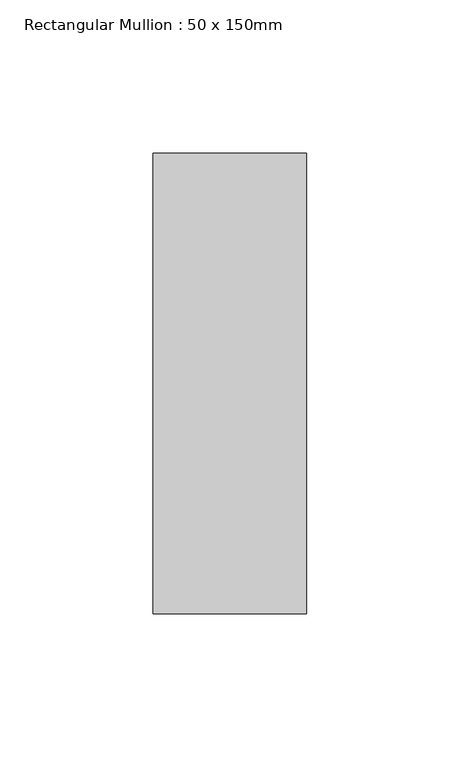
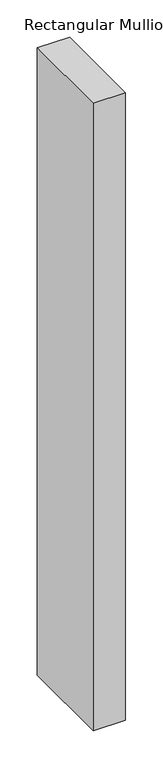
"""IFC4 building model written with IfcOpenShell, lengths in millimetres: member geometry, Rectangular Mullion : 50 x 150mm."""

from ifc_helpers import new_model, si_unit, frame, origin, place, context, project, spatial, polyline, outline, extrude, source, transform, mapped, element, save


def rectangular_mullion_50_x_150mm_37458a5b(model_context):
    return source(origin(), model_context, "Body", "SweptSolid", [
        extrude(outline(polyline([(0.0, 75.0), (0.0, -75.0), (-50.0, -75.0), (-50.0, 75.0), (0.0, 75.0)])), frame((0.0, 0.0, -1027.5595785), z_axis=(0.0, 0.0, 1.0), x_axis=(1.0, 0.0, 0.0)), (0.0, 0.0, 1.0), 1027.5595785),
    ])


if __name__ == "__main__":
    model = new_model("IFC4")
    model_context = context("Model", 3, world=origin())
    ifc_project = project(units=[si_unit("LENGTHUNIT", "METRE", prefix="MILLI")], contexts=[model_context])
    site = spatial("IfcSite", under=ifc_project)
    building = spatial("IfcBuilding", under=site)
    placement = place(None, origin())
    rectangular_mullion_50_x_150mm_shape = rectangular_mullion_50_x_150mm_37458a5b(model_context)
    element("IfcMember", 1, ObjectType="Rectangular Mullion : 50 x 150mm", at=placement, inside=building, context=model_context, shape_type="MappedRepresentation", body=[
        mapped(rectangular_mullion_50_x_150mm_shape, transform((0.0, 0.0, 0.0), x_axis=(1.0, 0.0, 0.0), y_axis=(0.0, 1.0, 0.0), z_axis=(0.0, 0.0, 1.0))),
    ])
    save(model, "model.ifc")

# Revit data of these elements
# Type "Rectangular Mullion : 50 x 150mm"
#   built-in parameter 1007304 = 0.492126 (stored number, unit not read)
#   built-in parameter 1007301 = 0.082021 (stored number, unit not read)
#   built-in parameter 1007300 = 0.082021 (stored number, unit not read)
# Element 1 (IfcMember, "Rectangular Mullion : 50 x 150mm")
#   Materials on its faces: "Aluminium"
# Materials
#   "Aluminium": class "Metal", colour RGB 247 247 247, transparency 0, Description = "Aluminium 6061", Cost = 0
